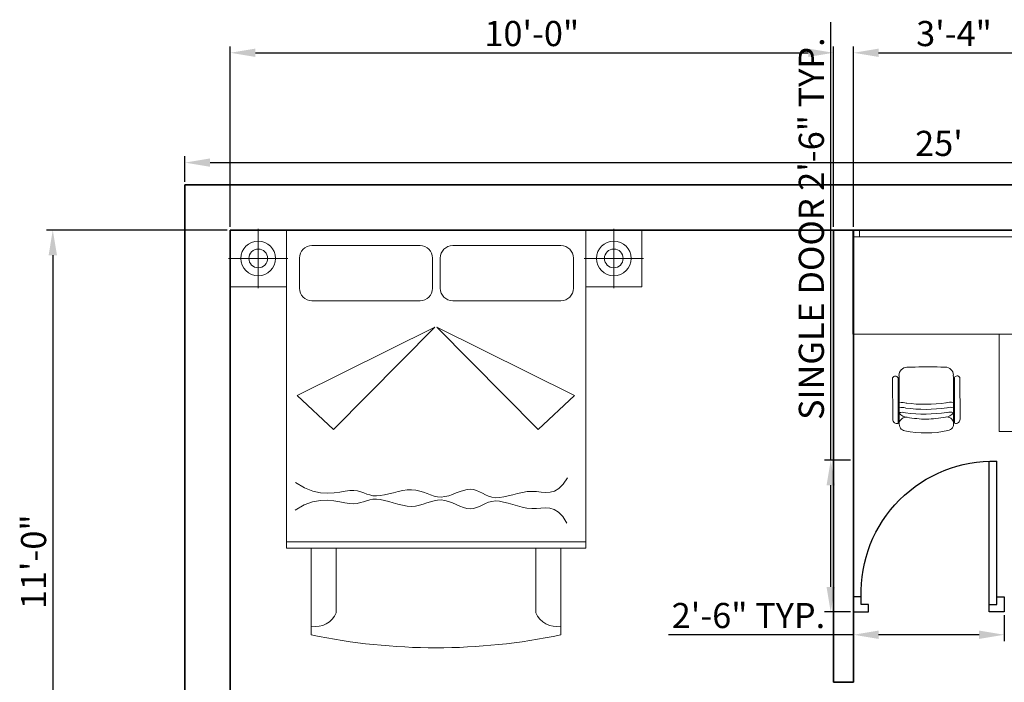
# Model space of a CAD drawing. Units: inches. Extents: x -24887 to 3061, y 1794 to 4919553.
# Tile 6 of 14: x 2132 to 2328, y 2218 to 2350. Entities that reach past the tile are written whole.
import ezdxf

# ---------------------------------------------------------------- set-up
doc = ezdxf.new("R2010")
doc.units = ezdxf.units.IN
for name, color, linetype, lineweight in [('A-ANNO-DIMS', 2, 'Continuous', 18), ('A-FURN', 8, 'Continuous', 18), ('door', 4, 'Continuous', 25), ('wall', 7, 'Continuous', 35)]:
    doc.layers.add(name, color=color, linetype=linetype, lineweight=lineweight)
doc.styles.get("Standard").update_dxf_attribs({"font": 'arial.ttf'})
doc.dimstyles.new('ISO-25', dxfattribs={"dimtxt": 5, "dimasz": 5, "dimexe": 1.25, "dimexo": 0.625, "dimtad": 1, "dimdec": 1, "dimlunit": 3, "dimtxsty": 'Standard', "dimcen": 2.5, "dimadec": 0, "dimazin": 0, "dimtfac": 1, "dimtdec": 1, "dimtmove": 0, "dimatfit": 3, "dimfxl": 1, "dimarcsym": 0})

# ---------------------------------------------------------------- blocks, each defined once
blk = doc.blocks.new('A$C4F543DC7')
for p, q in [((0.0134, 3.35, -0.1688), (3.3134, 3.35, -0.1688)), ((0.4634, 3.35, -0.1688), (0.0134, 3.35, -0.1688)), ((0.0134, 2.896, -0.1688), (0.0134, 3.35, -0.1688)), ((0.0134, 3.35, -0.1688), (0.0134, 2.896, -0.1688)), ((0.2381, 3.1233, -0.4388), (0.2381, 3.3614, -0.4388)), ((0.4634, 3.35, -0.1688), (0.4634, 0.8, -0.1688)), ((2.8634, 3.35, -0.1688), (0.4634, 3.35, -0.1688)), ((0.4634, 2.896, -0.1688), (0.4634, 3.35, -0.1688)), ((2.8634, 0.8, -0.1688), (2.8634, 3.35, -0.1688)), ((2.8634, 3.35, -0.1688), (3.3134, 3.35, -0.1688)), ((2.8634, 2.896, -0.1688), (2.8634, 3.35, -0.1688)), ((3.0888, 3.1233, -0.4388), (3.0888, 3.3614, -0.4388)), ((3.3134, 3.35, -0.1688), (3.3134, 2.896, -0.1688)), ((3.3134, 3.35, -0.1688), (3.3134, 2.896, -0.1688)), ((1.5354, 3.226, -0.1688), (0.6684, 3.226, -0.1688)), ((2.6644, 3.226, -0.1688), (1.7974, 3.226, -0.1688)), ((0.2381, 3.1233, -0.4388), (0, 3.1233, -0.4388)), ((0.2381, 3.1233, -0.4388), (0.4762, 3.1233, -0.4388)), ((0.2381, 3.1233, -0.4388), (0.2381, 2.8852, -0.4388)), ((0.5684, 3.126, -0.1688), (0.5684, 2.884, -0.1688)), ((1.6354, 2.884, -0.1688), (1.6354, 3.126, -0.1688)), ((1.6974, 3.126, -0.1688), (1.6974, 2.884, -0.1688)), ((2.7644, 2.884, -0.1688), (2.7644, 3.126, -0.1688)), ((3.0888, 3.1233, -0.4388), (2.8507, 3.1233, -0.4388)), ((3.0888, 3.1233, -0.4388), (3.0888, 2.8852, -0.4388)), ((3.0888, 3.1233, -0.4388), (3.3269, 3.1233, -0.4388)), ((0.4634, 2.896, -0.1688), (0.0134, 2.896, -0.1688)), ((0.0134, 2.896, -0.1688), (0.4634, 2.896, -0.1688)), ((0.4634, 0.8, -0.1688), (0.4634, 2.896, -0.1688)), ((2.8634, 2.896, -0.1688), (2.8634, 0.8, -0.1688)), ((3.3134, 2.896, -0.1688), (2.8634, 2.896, -0.1688)), ((3.3134, 2.896, -0.1688), (2.8634, 2.896, -0.1688)), ((0.6684, 2.784, -0.1688), (1.5354, 2.784, -0.1688)), ((1.7974, 2.784, -0.1688), (2.6644, 2.784, -0.1688)), ((1.6534, 2.573, -0.1688), (0.5504, 2.025, -0.1688)), ((0.8414, 1.752, -0.1688), (1.6534, 2.573, -0.1688)), ((2.4814, 1.752, -0.1688), (1.6694, 2.573, -0.1688)), ((1.6694, 2.573, -0.1688), (2.7724, 2.025, -0.1688)), ((0.5504, 2.025, -0.1688), (0.8414, 1.752, -0.1688)), ((2.7724, 2.025, -0.1688), (2.4814, 1.752, -0.1688)), ((2.683, 1.312, -0.1688), (2.7182, 1.3641, -0.1688)), ((0.5369, 1.3267, -0.1688), (0.6088, 1.2835, -0.1688)), ((0.6088, 1.2835, -0.1688), (0.6756, 1.2566, -0.1688)), ((1.3963, 1.2612, -0.1688), (1.4328, 1.2664, -0.1688)), ((1.4328, 1.2664, -0.1688), (1.4679, 1.2677, -0.1688)), ((1.4679, 1.2677, -0.1688), (1.501, 1.2643, -0.1688)), ((1.501, 1.2643, -0.1688), (1.5324, 1.257, -0.1688)), ((1.8849, 1.263, -0.1688), (1.913, 1.2698, -0.1688)), ((1.913, 1.2698, -0.1688), (1.9397, 1.2722, -0.1688)), ((1.9397, 1.2722, -0.1688), (1.9649, 1.2692, -0.1688)), ((1.9649, 1.2692, -0.1688), (1.989, 1.2617, -0.1688)), ((2.6129, 1.257, -0.1688), (2.6479, 1.2774, -0.1688)), ((2.6479, 1.2774, -0.1688), (2.683, 1.312, -0.1688)), ((0.6756, 1.2566, -0.1688), (0.7373, 1.2428, -0.1688)), ((0.7364, 1.1825, -0.1688), (0.7931, 1.1846, -0.1688)), ((0.7373, 1.2428, -0.1688), (0.794, 1.239, -0.1688)), ((0.7931, 1.1846, -0.1688), (0.8447, 1.1799, -0.1688)), ((0.794, 1.239, -0.1688), (0.8457, 1.242, -0.1688)), ((0.8457, 1.242, -0.1688), (0.8925, 1.2489, -0.1688)), ((0.8925, 1.2489, -0.1688), (0.9345, 1.2564, -0.1688)), ((0.9345, 1.2564, -0.1688), (0.9718, 1.2615, -0.1688)), ((0.9718, 1.2615, -0.1688), (1.0044, 1.2617, -0.1688)), ((1.0044, 1.2617, -0.1688), (1.0334, 1.2578, -0.1688)), ((1.0334, 1.2578, -0.1688), (1.0597, 1.2509, -0.1688)), ((1.0597, 1.2509, -0.1688), (1.0842, 1.2424, -0.1688)), ((1.0842, 1.2424, -0.1688), (1.1081, 1.2336, -0.1688)), ((1.1072, 1.18, -0.1688), (1.1316, 1.1872, -0.1688)), ((1.1081, 1.2336, -0.1688), (1.1322, 1.2257, -0.1688)), ((1.1316, 1.1872, -0.1688), (1.1573, 1.192, -0.1688)), ((1.1322, 1.2257, -0.1688), (1.1577, 1.2201, -0.1688)), ((1.1573, 1.192, -0.1688), (1.1851, 1.1932, -0.1688)), ((1.1577, 1.2201, -0.1688), (1.1855, 1.218, -0.1688)), ((1.1851, 1.1932, -0.1688), (1.2158, 1.1898, -0.1688)), ((1.1855, 1.218, -0.1688), (1.2163, 1.2204, -0.1688)), ((1.2158, 1.1898, -0.1688), (1.2491, 1.1828, -0.1688)), ((1.2163, 1.2204, -0.1688), (1.2498, 1.2264, -0.1688)), ((1.2498, 1.2264, -0.1688), (1.2852, 1.2347, -0.1688)), ((1.2852, 1.2347, -0.1688), (1.3218, 1.2441, -0.1688)), ((1.3218, 1.2441, -0.1688), (1.3591, 1.2533, -0.1688)), ((1.3591, 1.2533, -0.1688), (1.3963, 1.2612, -0.1688)), ((1.5324, 1.257, -0.1688), (1.5624, 1.2473, -0.1688)), ((1.5624, 1.2473, -0.1688), (1.5915, 1.2365, -0.1688)), ((1.5915, 1.2365, -0.1688), (1.6199, 1.2259, -0.1688)), ((1.6199, 1.2259, -0.1688), (1.6481, 1.2169, -0.1688)), ((1.6475, 1.1797, -0.1688), (1.676, 1.1849, -0.1688)), ((1.6481, 1.2169, -0.1688), (1.6765, 1.2108, -0.1688)), ((1.676, 1.1849, -0.1688), (1.7049, 1.1858, -0.1688)), ((1.6765, 1.2108, -0.1688), (1.7053, 1.209, -0.1688)), ((1.7049, 1.1858, -0.1688), (1.7344, 1.1816, -0.1688)), ((1.7053, 1.209, -0.1688), (1.7349, 1.2124, -0.1688)), ((1.7349, 1.2124, -0.1688), (1.7651, 1.2199, -0.1688)), ((1.7651, 1.2199, -0.1688), (1.7955, 1.2301, -0.1688)), ((1.7955, 1.2301, -0.1688), (1.8258, 1.2417, -0.1688)), ((1.8258, 1.2417, -0.1688), (1.8557, 1.2531, -0.1688)), ((1.8557, 1.2531, -0.1688), (1.8849, 1.263, -0.1688)), ((1.989, 1.2617, -0.1688), (2.0124, 1.2512, -0.1688)), ((2.0124, 1.2512, -0.1688), (2.0359, 1.2391, -0.1688)), ((2.0359, 1.2391, -0.1688), (2.0599, 1.2269, -0.1688)), ((2.0599, 1.2269, -0.1688), (2.0849, 1.216, -0.1688)), ((2.0849, 1.216, -0.1688), (2.1117, 1.2077, -0.1688)), ((2.1117, 1.2077, -0.1688), (2.1407, 1.2037, -0.1688)), ((2.1407, 1.2037, -0.1688), (2.1723, 1.2047, -0.1688)), ((2.1723, 1.2047, -0.1688), (2.2062, 1.21, -0.1688)), ((2.2062, 1.21, -0.1688), (2.242, 1.2182, -0.1688)), ((2.242, 1.2182, -0.1688), (2.2791, 1.2279, -0.1688)), ((2.2791, 1.2279, -0.1688), (2.3173, 1.2378, -0.1688)), ((2.3173, 1.2378, -0.1688), (2.3558, 1.2465, -0.1688)), ((2.3558, 1.2465, -0.1688), (2.3944, 1.2527, -0.1688)), ((2.3944, 1.2527, -0.1688), (2.4325, 1.255, -0.1688)), ((2.4325, 1.255, -0.1688), (2.4698, 1.2529, -0.1688)), ((2.4698, 1.2529, -0.1688), (2.5064, 1.2488, -0.1688)), ((2.5064, 1.2488, -0.1688), (2.5423, 1.2459, -0.1688)), ((2.5423, 1.2459, -0.1688), (2.5777, 1.2476, -0.1688)), ((2.5777, 1.2476, -0.1688), (2.6129, 1.257, -0.1688)), ((0.5334, 1.105, -0.1688), (0.6067, 1.1458, -0.1688)), ((0.6067, 1.1458, -0.1688), (0.6743, 1.1706, -0.1688)), ((0.6743, 1.1706, -0.1688), (0.7364, 1.1825, -0.1688)), ((0.8447, 1.1799, -0.1688), (0.8913, 1.1716, -0.1688)), ((0.8913, 1.1716, -0.1688), (0.9331, 1.1628, -0.1688)), ((0.9331, 1.1628, -0.1688), (0.9701, 1.1565, -0.1688)), ((0.9701, 1.1565, -0.1688), (1.0027, 1.1552, -0.1688)), ((1.0027, 1.1552, -0.1688), (1.0318, 1.1582, -0.1688)), ((1.0318, 1.1582, -0.1688), (1.0583, 1.1642, -0.1688)), ((1.0583, 1.1642, -0.1688), (1.0831, 1.172, -0.1688)), ((1.0831, 1.172, -0.1688), (1.1072, 1.18, -0.1688)), ((1.2491, 1.1828, -0.1688), (1.2842, 1.1734, -0.1688)), ((1.2842, 1.1734, -0.1688), (1.3206, 1.1629, -0.1688)), ((1.3206, 1.1629, -0.1688), (1.3575, 1.1524, -0.1688)), ((1.3575, 1.1524, -0.1688), (1.3945, 1.1434, -0.1688)), ((1.3945, 1.1434, -0.1688), (1.4308, 1.1371, -0.1688)), ((1.4308, 1.1371, -0.1688), (1.4658, 1.1347, -0.1688)), ((1.4658, 1.1347, -0.1688), (1.499, 1.137, -0.1688)), ((1.499, 1.137, -0.1688), (1.5306, 1.1433, -0.1688)), ((1.5306, 1.1433, -0.1688), (1.5609, 1.152, -0.1688)), ((1.5609, 1.152, -0.1688), (1.5903, 1.1619, -0.1688)), ((1.5903, 1.1619, -0.1688), (1.6191, 1.1716, -0.1688)), ((1.6191, 1.1716, -0.1688), (1.6475, 1.1797, -0.1688)), ((1.7344, 1.1816, -0.1688), (1.7643, 1.1731, -0.1688)), ((1.7643, 1.1731, -0.1688), (1.7944, 1.1619, -0.1688)), ((1.7944, 1.1619, -0.1688), (1.8244, 1.1494, -0.1688)), ((1.8244, 1.1494, -0.1688), (1.8539, 1.137, -0.1688)), ((1.8539, 1.137, -0.1688), (1.8827, 1.1263, -0.1688)), ((1.8827, 1.1263, -0.1688), (1.9106, 1.1186, -0.1688)), ((1.9106, 1.1186, -0.1688), (1.9373, 1.1153, -0.1688)), ((1.9373, 1.1153, -0.1688), (1.9625, 1.1176, -0.1688)), ((1.9625, 1.1176, -0.1688), (1.9868, 1.1243, -0.1688)), ((1.9868, 1.1243, -0.1688), (2.0106, 1.134, -0.1688)), ((2.0106, 1.134, -0.1688), (2.0344, 1.1454, -0.1688)), ((2.0344, 1.1454, -0.1688), (2.0588, 1.1568, -0.1688)), ((2.0588, 1.1568, -0.1688), (2.0842, 1.167, -0.1688)), ((2.0842, 1.167, -0.1688), (2.1112, 1.1743, -0.1688)), ((2.1112, 1.1743, -0.1688), (2.1403, 1.1775, -0.1688)), ((2.1403, 1.1775, -0.1688), (2.1718, 1.1755, -0.1688)), ((2.1718, 1.1755, -0.1688), (2.2056, 1.1691, -0.1688)), ((2.2056, 1.1691, -0.1688), (2.2411, 1.1598, -0.1688)), ((2.2411, 1.1598, -0.1688), (2.2779, 1.1489, -0.1688)), ((2.2779, 1.1489, -0.1688), (2.3157, 1.1379, -0.1688)), ((2.3157, 1.1379, -0.1688), (2.354, 1.1279, -0.1688)), ((2.354, 1.1279, -0.1688), (2.3923, 1.1205, -0.1688)), ((2.3923, 1.1205, -0.1688), (2.4304, 1.117, -0.1688)), ((2.4304, 1.117, -0.1688), (2.4677, 1.118, -0.1688)), ((2.4677, 1.118, -0.1688), (2.5043, 1.1209, -0.1688)), ((2.5043, 1.1209, -0.1688), (2.5403, 1.1226, -0.1688)), ((2.5403, 1.1226, -0.1688), (2.5757, 1.1199, -0.1688)), ((2.5757, 1.1199, -0.1688), (2.6106, 1.1094, -0.1688)), ((2.6106, 1.1094, -0.1688), (2.645, 1.0879, -0.1688)), ((2.645, 1.0879, -0.1688), (2.6789, 1.0522, -0.1688)), ((2.6789, 1.0522, -0.1688), (2.7124, 0.999, -0.1688)), ((0.4634, 0.85, -0.1688), (2.8634, 0.85, -0.1688)), ((0.4634, 0.8, -0.1688), (2.8634, 0.8, -0.1688)), ((0.6634, 0.8, -0.1688), (0.4634, 0.8, -0.1688)), ((0.6634, 0.8, -0.1688), (2.6634, 0.8, -0.1688)), ((0.6634, 0.104, -0.1688), (0.6634, 0.8, -0.1688)), ((0.6634, 0.104, -0.1688), (0.6634, 0.8, -0.1688)), ((0.8634, 0.281, -0.1688), (0.8634, 0.8, -0.1688)), ((2.4634, 0.8, -0.1688), (2.4634, 0.281, -0.1688)), ((2.8634, 0.8, -0.1688), (2.6634, 0.8, -0.1688)), ((2.6634, 0.8, -0.1688), (2.6634, 0.104, -0.1688)), ((2.6634, 0.8, -0.1688), (2.6634, 0.104, -0.1688))]:
    blk.add_line(p, q)
for centre, radius in [((0.2381, 3.1233, -0.4388), 0.139), ((3.0888, 3.1233, -0.4388), 0.139), ((0.2381, 3.1233, -0.4388), 0.075), ((3.0888, 3.1233, -0.4388), 0.075)]:
    blk.add_circle(centre, radius)
for centre, radius, start, end in [((0.6684, 3.126, -0.1688), 0.1, 90, 180), ((1.5354, 3.126, -0.1688), 0.1, 0, 90), ((1.7974, 3.126, -0.1688), 0.1, 90, 180), ((2.6644, 3.126, -0.1688), 0.1, 0, 90), ((0.6684, 2.884, -0.1688), 0.1, 180, 270), ((1.5354, 2.884, -0.1688), 0.1, 270, 0), ((1.7974, 2.884, -0.1688), 0.1, 180, 270), ((2.6644, 2.884, -0.1688), 0.1, 270, 0), ((0.6994, 0.3472, -0.1688), 0.1769, 258.2616, 338.03196), ((2.6275, 0.3472, -0.1688), 0.1769, 201.96804, 281.7384), ((1.6634, 4.8597, -0.1688), 4.8597, 258.12517, 281.87483), ((1.6634, 4.8597, -0.1688), 4.8597, 258.12517, 281.87483)]:
    blk.add_arc(centre, radius, start, end)
blk = doc.blocks.new('*D30')
at = {"layer": 'A-ANNO-DIMS', "color": 0, "lineweight": -2, "transparency": 16777216}
for p, q in [((2164.92, 2317.57), (2164.92, 2322.63)), ((2169.92, 2321.38), (2459.92, 2321.38)), ((2464.92, 2317.57), (2464.92, 2322.63))]:
    blk.add_line(p, q, dxfattribs=at)
at = {"layer": 'A-ANNO-DIMS', "color": 0, "transparency": 16777216}
for points in [[(2169.92, 2322.21), (2169.92, 2320.55), (2164.92, 2321.38)], [(2459.92, 2322.21), (2459.92, 2320.55), (2464.92, 2321.38)]]:
    blk.add_solid(points, dxfattribs=at)
at = {"layer": 'Defpoints', "color": 0, "transparency": 16777216}
for p in [(2464.92, 2321.38), (2164.92, 2316.94), (2464.92, 2316.94)]:
    blk.add_point(p, dxfattribs=at)
at = {"layer": 'A-ANNO-DIMS', "color": 0, "transparency": 16777216, "insert": (2314.92, 2324.56), "char_height": 5, "attachment_point": 5}
blk.add_mtext("25'", dxfattribs=at)
blk = doc.blocks.new('DESK-CORNER-WITH-CHAIR')
for p, q in [((0, 40.37), (40.11, 40.37)), ((0, 19.67), (0, 40.37)), ((1.29, 39.07), (1.29, 40.37)), ((38.82, 40.37), (38.82, 19.67)), ((40.11, 40.37), (40.11, 0.26)), ((0, 39.07), (40.11, 39.07)), ((38.82, 19.67), (0, 19.67)), ((29.11, 19.67), (38.82, 19.67)), ((29.11, 0.26), (29.11, 19.67)), ((38.82, 19.67), (38.82, 0.26)), ((10.75, 13.07), (10.91, 13.07)), ((11.62, 13.07), (10.91, 13.07)), ((17.49, 13.1), (18.37, 13.11)), ((7.89, 10.98), (7.93, 2.72)), ((8.97, 10.98), (9.02, 1.91)), ((9.17, 10.98), (9.17, 11.46)), ((9.17, 10.99), (9.18, 9.53)), ((19.98, 11.02), (19.97, 11.52)), ((19.98, 11.02), (19.98, 9.56)), ((20.18, 11.01), (20.22, 1.94)), ((21.26, 11.02), (21.3, 2.76)), ((9.17, 9.52), (9.22, 2.03)), ((19.99, 9.54), (20.03, 2.06)), ((40.11, 0.26), (29.11, 0.26)), ((40.11, 1.55), (38.82, 1.55))]:
    blk.add_line(p, q)
for centre, radius, start, end in [((10.76, 11.47), 1.6, 90.3083, 180.3083), ((14.78, -28.11), 41.3, 86.2317, 94.3849), ((18.38, 11.51), 1.6, 0.3083, 90.3083), ((8.43, 10.73), 0.593, 24.5958, 155.829), ((20.52, 10.77), 0.593, 204.3355, 206.5711), ((20.72, 10.77), 0.593, 24.7876, 156.0208), ((9.82, 2.64), 3.42, 74.7531, 100.4859), ((14.4, 34.16), 28.46, 262.2773, 278.3393), ((19.33, 2.69), 3.42, 78.6001, 104.4332), ((9.82, 2.64), 2.42, 74.7531, 104.4332), ((9.82, 1.7), 2.42, 74.7531, 104.4332), ((14.4, 34.16), 29.46, 262.2773, 278.3393), ((14.4, 33.22), 29.46, 262.2773, 278.3393), ((18.3, 5.37), 2.21, 273.1318, 320.9947), ((19.33, 2.69), 2.42, 73.6429, 104.4332), ((19.33, 1.75), 2.42, 73.6429, 104.4332), ((8.75, 2.68), 0.821, 177.6524, 288.8331), ((10.57, 1.77), 1.37, 80.5561, 260.4095), ((10.9, 5.33), 2.21, 220.0354, 267.4848), ((14.95, 25.37), 22.63, 259.4369, 269.1516), ((14.03, 25.37), 22.63, 271.465, 281.1797), ((18.66, 1.82), 1.37, 280.2071, 100.0605), ((20.48, 2.72), 0.821, 251.7835, 2.9643), ((14.52, 20.73), 20.73, 258.3982, 282.2184)]:
    blk.add_arc(centre, radius, start, end)
blk = doc.blocks.new('DOOR-SINGLE-30IN')
for p, q in [((1.5, 1.5), (1.5, 30)), ((3, 0), (3, 30)), ((0, 3), (0, 0)), ((1.5, 3), (0, 3)), ((1.5, 1.5), (1.5, 3)), ((28.5, 1.5), (28.5, 3)), ((28.5, 3), (30, 3)), ((30, 3), (30, 0)), ((0, 0), (3, 0)), ((3, 1.5), (1.5, 1.5)), ((3, 0), (3, 1.5)), ((27, 0), (27, 1.5)), ((27, 1.5), (28.5, 1.5)), ((30, 0), (27, 0))]:
    blk.add_line(p, q)
blk.add_arc((2.25, 3.75), 26.26, 358.3634, 91.6366)
blk = doc.blocks.new('*D56')
at = {"layer": 'A-ANNO-DIMS', "color": 0, "lineweight": -2, "transparency": 16777216}
for p, q in [((2293.39, 2262.15), (2293.39, 2349.31)), ((2297.3, 2262.15), (2292.14, 2262.15)), ((2293.39, 2236.94), (2293.39, 2257.15)), ((2297.3, 2231.94), (2292.14, 2231.94))]:
    blk.add_line(p, q, dxfattribs=at)
at = {"layer": 'A-ANNO-DIMS', "color": 0, "transparency": 16777216}
for points in [[(2292.56, 2257.15), (2294.23, 2257.15), (2293.39, 2262.15)], [(2292.56, 2236.94), (2294.23, 2236.94), (2293.39, 2231.94)]]:
    blk.add_solid(points, dxfattribs=at)
at = {"layer": 'Defpoints', "color": 0, "transparency": 16777216}
for p in [(2293.39, 2262.15), (2297.92, 2262.15), (2297.92, 2231.94)]:
    blk.add_point(p, dxfattribs=at)
at = {"layer": 'A-ANNO-DIMS', "color": 0, "transparency": 16777216, "insert": (2290.18, 2308.23), "char_height": 5, "attachment_point": 5, "rotation": 90}
blk.add_mtext('SINGLE DOOR 2\'-6" TYP.', dxfattribs=at)
blk = doc.blocks.new('*D57')
at = {"layer": 'A-ANNO-DIMS', "color": 0, "lineweight": -2, "transparency": 16777216}
for p, q in [((2297.92, 2231.32), (2297.92, 2226.16)), ((2327.92, 2231.32), (2327.92, 2226.16)), ((2297.92, 2227.41), (2261.11, 2227.41)), ((2322.92, 2227.41), (2302.92, 2227.41))]:
    blk.add_line(p, q, dxfattribs=at)
at = {"layer": 'A-ANNO-DIMS', "color": 0, "transparency": 16777216}
for points in [[(2302.92, 2228.24), (2302.92, 2226.58), (2297.92, 2227.41)], [(2322.92, 2228.24), (2322.92, 2226.58), (2327.92, 2227.41)]]:
    blk.add_solid(points, dxfattribs=at)
at = {"layer": 'Defpoints', "color": 0, "transparency": 16777216}
for p in [(2297.92, 2231.94), (2327.92, 2231.94), (2297.92, 2227.41)]:
    blk.add_point(p, dxfattribs=at)
at = {"layer": 'A-ANNO-DIMS', "color": 0, "transparency": 16777216, "insert": (2277.02, 2230.59), "char_height": 5, "attachment_point": 5}
blk.add_mtext('2\'-6" TYP.', dxfattribs=at)
blk = doc.blocks.new('*D83')
at = {"layer": 'A-ANNO-DIMS', "color": 0, "lineweight": -2, "transparency": 16777216}
for p, q in [((2173.92, 2308.57), (2173.92, 2344.49)), ((2178.92, 2343.24), (2288.92, 2343.24)), ((2293.92, 2308.57), (2293.92, 2344.49))]:
    blk.add_line(p, q, dxfattribs=at)
at = {"layer": 'A-ANNO-DIMS', "color": 0, "transparency": 16777216}
for points in [[(2178.92, 2344.07), (2178.92, 2342.41), (2173.92, 2343.24)], [(2288.92, 2344.07), (2288.92, 2342.41), (2293.92, 2343.24)]]:
    blk.add_solid(points, dxfattribs=at)
at = {"layer": 'Defpoints', "color": 0, "transparency": 16777216}
for p in [(2293.92, 2343.24), (2173.92, 2307.94), (2293.92, 2307.94)]:
    blk.add_point(p, dxfattribs=at)
at = {"layer": 'A-ANNO-DIMS', "color": 0, "transparency": 16777216, "insert": (2233.92, 2346.42), "char_height": 5, "attachment_point": 5}
blk.add_mtext('10\'-0"', dxfattribs=at)
blk = doc.blocks.new('*D84')
at = {"layer": 'A-ANNO-DIMS', "color": 0, "lineweight": -2, "transparency": 16777216}
for p, q in [((2297.92, 2308.57), (2297.92, 2344.49)), ((2302.92, 2343.24), (2332.92, 2343.24)), ((2337.92, 2308.57), (2337.92, 2344.49))]:
    blk.add_line(p, q, dxfattribs=at)
at = {"layer": 'A-ANNO-DIMS', "color": 0, "transparency": 16777216}
for points in [[(2302.92, 2344.07), (2302.92, 2342.41), (2297.92, 2343.24)], [(2332.92, 2344.07), (2332.92, 2342.41), (2337.92, 2343.24)]]:
    blk.add_solid(points, dxfattribs=at)
at = {"layer": 'Defpoints', "color": 0, "transparency": 16777216}
for p in [(2337.92, 2343.24), (2297.92, 2307.94), (2337.92, 2307.94)]:
    blk.add_point(p, dxfattribs=at)
at = {"layer": 'A-ANNO-DIMS', "color": 0, "transparency": 16777216, "insert": (2317.92, 2346.42), "char_height": 5, "attachment_point": 5}
blk.add_mtext('3\'-4"', dxfattribs=at)
blk = doc.blocks.new('*D88')
at = {"layer": 'A-ANNO-DIMS', "color": 0, "lineweight": -2, "transparency": 16777216}
for p, q in [((2173.3, 2307.94), (2137.37, 2307.94)), ((2138.62, 2302.94), (2138.62, 2180.94)), ((2173.3, 2175.94), (2137.37, 2175.94))]:
    blk.add_line(p, q, dxfattribs=at)
at = {"layer": 'A-ANNO-DIMS', "color": 0, "transparency": 16777216}
for points in [[(2137.79, 2302.94), (2139.46, 2302.94), (2138.62, 2307.94)], [(2137.79, 2180.94), (2139.46, 2180.94), (2138.62, 2175.94)]]:
    blk.add_solid(points, dxfattribs=at)
at = {"layer": 'Defpoints', "color": 0, "transparency": 16777216}
for p in [(2173.92, 2307.94), (2138.62, 2175.94), (2173.92, 2175.94)]:
    blk.add_point(p, dxfattribs=at)
at = {"layer": 'A-ANNO-DIMS', "color": 0, "transparency": 16777216, "insert": (2135.45, 2241.94), "char_height": 5, "attachment_point": 5, "rotation": 90}
blk.add_mtext('11\'-0"', dxfattribs=at)

msp = doc.modelspace()

# ---------------------------------------------------------------- linework, layer by layer
at = {"layer": 'wall'}
for p, q in [((2464.92, 2316.94), (2164.92, 2316.94)), ((2164.92, 2316.94), (2164.92, 1956.94)), ((2455.92, 2307.94), (2173.92, 2307.94)), ((2173.92, 2307.94), (2173.92, 1965.94)), ((2293.92, 2307.94), (2293.92, 2217.94)), ((2297.92, 2307.94), (2297.92, 2235.94)), ((2297.92, 2235.94), (2297.92, 2231.94)), ((2297.92, 2231.94), (2297.92, 2217.94)), ((2293.92, 2217.94), (2297.92, 2217.94))]:
    msp.add_line(p, q, dxfattribs=at)

# ---------------------------------------------------------------- block references
at = {"layer": 'A-FURN', "xscale": 24.81469674658305, "yscale": 24.81469674658305, "zscale": 24.81469674658305}
msp.add_blockref('A$C4F543DC7', (2173.59, 2224.81, 4.19), dxfattribs=at)
at = {"layer": 'A-FURN'}
msp.add_blockref('DESK-CORNER-WITH-CHAIR', (2297.81, 2267.57), dxfattribs=at)
at = {"layer": 'door', "extrusion": (0, 0, -1), "zscale": -1}
msp.add_blockref('DOOR-SINGLE-30IN', (-2327.92, 2231.94), dxfattribs=at)

# ---------------------------------------------------------------- dimensions: what is measured, and where the dimension line sits
at = {"layer": 'A-ANNO-DIMS'}
for base, p1, p2, override, picture, middle in [((2293.92, 2343.24), (2173.92, 2307.94), (2293.92, 2307.94), {"dimdec": 1, "dimlfac": 1, "dimrnd": 0, "dimzin": 1, "dimdsep": 46, "dimlunit": 4, "dimfrac": 2}, '*D83', (2233.92, 2346.42)), ((2337.92, 2343.24), (2297.92, 2307.94), (2337.92, 2307.94), {"dimdec": 1, "dimlfac": 1, "dimrnd": 0, "dimzin": 1, "dimdsep": 46, "dimlunit": 4, "dimfrac": 2}, '*D84', (2317.92, 2346.42)), ((2464.92, 2321.38), (2164.92, 2316.94), (2464.92, 2316.94), {"dimclrd": 0, "dimclre": 0, "dimclrt": 0}, '*D30', (2314.92, 2324.56))]:
    dim = msp.add_linear_dim(base=base, p1=p1, p2=p2, dimstyle='ISO-25', override=override, dxfattribs=at)
    dim.commit()
    dim.dimension.update_dxf_attribs({"geometry": picture, "text_midpoint": middle})
for base, p1, p2, angle, text, picture, middle in [((2293.39, 2262.15), (2297.92, 2231.94), (2297.92, 2262.15), 90, 'SINGLE DOOR <> TYP.', '*D56', (2290.18, 2308.23)), ((2297.92, 2227.41), (2327.92, 2231.94), (2297.92, 2231.94), 180, '<> TYP.', '*D57', (2277.02, 2230.59))]:
    dim = msp.add_linear_dim(base=base, p1=p1, p2=p2, angle=angle, text=text, dimstyle='ISO-25', override={"dimdec": 1, "dimlfac": 1, "dimrnd": 0, "dimzin": 1, "dimdsep": 46, "dimlunit": 4, "dimfrac": 2}, dxfattribs=at)
    dim.commit()
    dim.dimension.update_dxf_attribs({"geometry": picture, "text_midpoint": middle})
dim = msp.add_linear_dim(base=(2138.62, 2175.94), p1=(2173.92, 2307.94), p2=(2173.92, 2175.94), angle=90, dimstyle='ISO-25', override={"dimdec": 1, "dimlfac": 1, "dimrnd": 0, "dimzin": 1, "dimdsep": 46, "dimlunit": 4, "dimfrac": 2}, dxfattribs=at)
dim.commit()
dim.dimension.update_dxf_attribs({"geometry": '*D88', "text_midpoint": (2135.45, 2241.94)})

doc.saveas('drawing.dxf')
